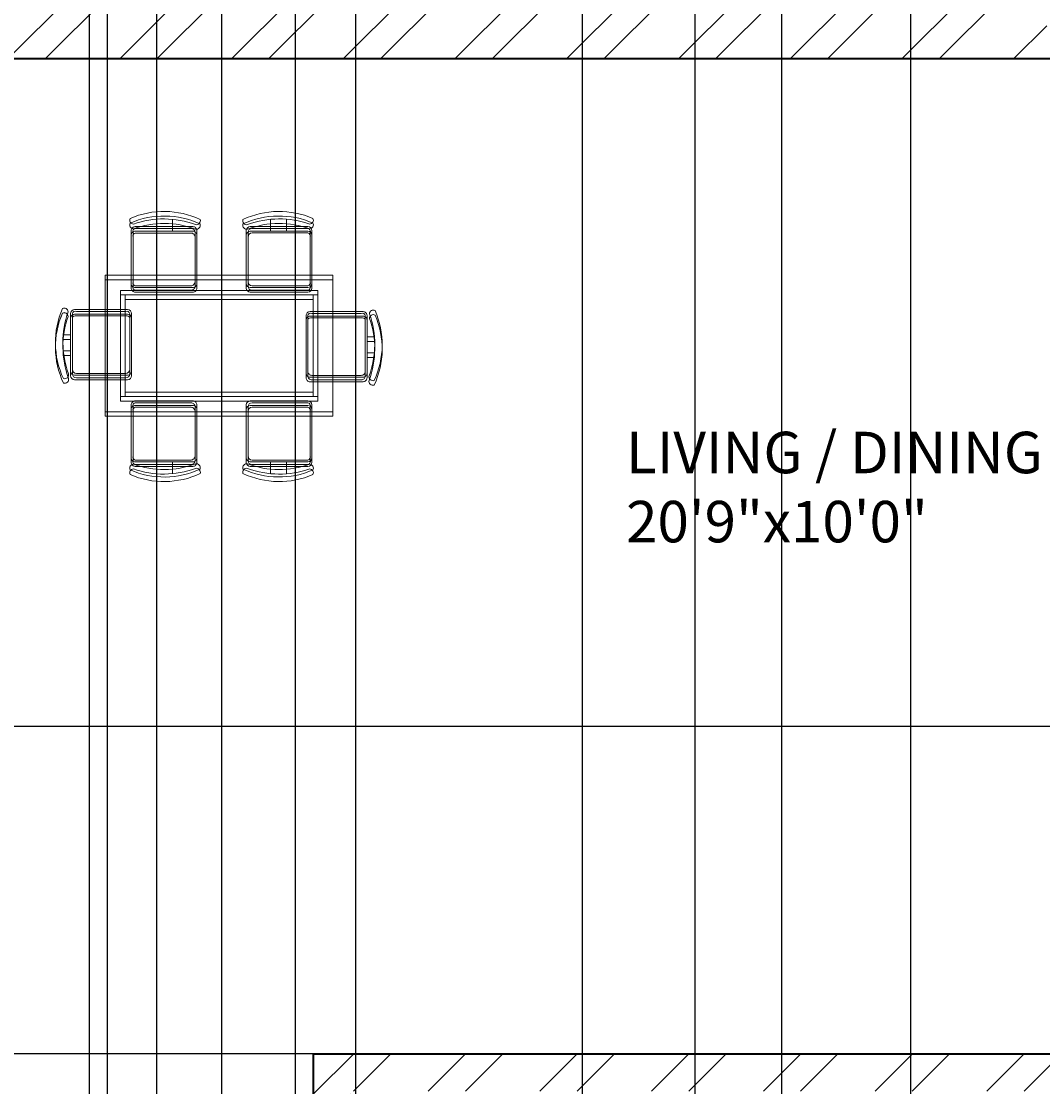
# Model space of a CAD drawing. Units: inches. Extents: x 1748 to 2382, y 1346 to 2284.
# Tile 6 of 26: x 2024 to 2147, y 1602 to 1730. Entities that reach past the tile are written whole.
import ezdxf

# ---------------------------------------------------------------- set-up
doc = ezdxf.new("R2010")
doc.units = ezdxf.units.IN
for name, color, linetype, lineweight in [('A-ANNO-DIMS', 2, 'Continuous', 18), ('A-AREA-IDEN', 7, 'Continuous', 18), ('A-FURN', 8, 'Continuous', 13), ('A-WALL', 7, 'Continuous', 35), ('A-WALL-PATT', 9, 'Continuous', 13)]:
    doc.layers.add(name, color=color, linetype=linetype, lineweight=lineweight)
doc.styles.get("Standard").update_dxf_attribs({"font": 'arial.ttf'})
doc.dimstyles.get("Standard").update_dxf_attribs({"dimtxt": 0.18, "dimasz": 0.18, "dimexe": 0.18, "dimexo": 0.0625, "dimgap": 0.09, "dimtad": 0, "dimtih": 1, "dimtoh": 1, "dimdec": 4, "dimzin": 0, "dimdsep": 46, "dimtxsty": 'Standard', "dimcen": 0.09, "dimadec": 0, "dimazin": 0, "dimtfac": 1, "dimtdec": 4, "dimtofl": 0, "dimtmove": 0, "dimatfit": 3, "dimfxl": 1, "dimtolj": 1, "dimtzin": 0, "dimarcsym": 0})

# ---------------------------------------------------------------- blocks, each defined once
blk = doc.blocks.new('TABLE-DINING')
for points in [[(0, 17.02), (27.45, 17.02), (27.45, 0.55), (0, 0.55)], [(0, 17.02), (27.45, 17.02), (27.45, 0.55), (0, 0.55)], [(0, 16.47), (27.45, 16.47), (27.45, 0), (0, 0)], [(0, 16.47), (27.45, 16.47), (27.45, 0), (0, 0)], [(1.83, 15.19), (25.62, 15.19), (25.62, 2.38), (1.83, 2.38)], [(1.83, 15.19), (25.62, 15.19), (25.62, 2.38), (1.83, 2.38)], [(1.83, 14.64), (25.62, 14.64), (25.62, 1.83), (1.83, 1.83)], [(1.83, 14.64), (25.62, 14.64), (25.62, 1.83), (1.83, 1.83)], [(2.38, 14.64), (25.07, 14.64), (25.07, 2.93), (2.38, 2.93)], [(2.38, 14.64), (25.07, 14.64), (25.07, 2.93), (2.38, 2.93)], [(2.38, 14.09), (25.07, 14.09), (25.07, 2.38), (2.38, 2.38)], [(2.38, 14.09), (25.07, 14.09), (25.07, 2.38), (2.38, 2.38)]]:
    blk.add_lwpolyline(points, close=True)
blk = doc.blocks.new('CHAIR-DINING-SIDE')
for points in [[(0.45, 8.2, -0.175809), (7.92, 8.14, 0.578392), (8.49, 8.77, 0.214524), (0.05, 8.88, 0.552014), (0.45, 8.2, -0.065079)], [(0.45, 8.2, -0.175809), (7.92, 8.14, 0.578392), (8.49, 8.77, 0.214524), (0.05, 8.88, 0.552014), (0.45, 8.2, -0.065079)], [(0.45, 7.65, -0.175809), (7.92, 7.6, 0.578392), (8.49, 8.22, 0.214524), (0.05, 8.33, 0.552014), (0.45, 7.65, -0.065079)], [(0.45, 7.65, -0.175809), (7.92, 7.6, 0.578392), (8.49, 8.22, 0.214524), (0.05, 8.33, 0.552014), (0.45, 7.65, -0.065079)], [(7.61, 7.9), (0.67, 7.9, 0.414214), (0.18, 7.42), (0.18, 1.03, 0.414214), (0.67, 0.55), (7.61, 0.55, 0.414214), (8.09, 1.03), (8.09, 7.42, 0.414214), (7.61, 7.9)], [(7.61, 7.9), (0.67, 7.9, 0.414214), (0.18, 7.42), (0.18, 1.03, 0.414214), (0.67, 0.55), (7.61, 0.55, 0.414214), (8.09, 1.03), (8.09, 7.42, 0.414214), (7.61, 7.9)], [(5.17, 7.9), (5.17, 8.78, -0.064759)], [(5.17, 7.9), (5.17, 8.78, -0.064759)], [(5.17, 7.35), (5.17, 8.23, -0.064759)], [(5.17, 7.35), (5.17, 8.23, -0.064759)], [(7.61, 7.35), (0.67, 7.35, 0.414214), (0.18, 6.87), (0.18, 0.49, 0.414214), (0.67, 0), (7.61, 0, 0.414214), (8.09, 0.49), (8.09, 6.87, 0.414214), (7.61, 7.35)], [(7.61, 7.35), (0.67, 7.35, 0.414214), (0.18, 6.87), (0.18, 0.49, 0.414214), (0.67, 0), (7.61, 0, 0.414214), (8.09, 0.49), (8.09, 6.87, 0.414214), (7.61, 7.35)]]:
    blk.add_lwpolyline(points, format="xyb")
for points in [[(3.23, 8.79), (3.23, 7.9)], [(3.23, 8.79), (3.23, 7.9)], [(3.23, 8.25), (3.23, 7.35)], [(3.23, 8.25), (3.23, 7.35)]]:
    blk.add_lwpolyline(points)
for points in [[(0.67, 7.68), (7.39, 7.68, -0.414214), (7.87, 7.2), (7.87, 1.25, -0.414214), (7.39, 0.77), (0.67, 0.77, -0.512069), (0.4, 1.25), (0.4, 7.2, -0.512069)], [(0.67, 7.68), (7.39, 7.68, -0.414214), (7.87, 7.2), (7.87, 1.25, -0.414214), (7.39, 0.77), (0.67, 0.77, -0.512069), (0.4, 1.25), (0.4, 7.2, -0.512069)], [(0.67, 7.13), (7.39, 7.13, -0.414214), (7.87, 6.65), (7.87, 0.7, -0.414214), (7.39, 0.22), (0.67, 0.22, -0.512069), (0.4, 0.7), (0.4, 6.65, -0.512069)], [(0.67, 7.13), (7.39, 7.13, -0.414214), (7.87, 6.65), (7.87, 0.7, -0.414214), (7.39, 0.22), (0.67, 0.22, -0.512069), (0.4, 0.7), (0.4, 6.65, -0.512069)]]:
    blk.add_lwpolyline(points, format="xyb", close=True)
blk = doc.blocks.new('CHAIR-DINING-END')
for points in [[(7.65, 8.61, -0.175809), (7.6, 1.14, 0.578392), (8.22, 0.57, 0.214524), (8.33, 9.01, 0.552014), (7.65, 8.61, -0.065079)], [(7.65, 8.61, -0.175809), (7.6, 1.14, 0.578392), (8.22, 0.57, 0.214524), (8.33, 9.01, 0.552014), (7.65, 8.61, -0.065079)], [(7.35, 8.4, 0.414214), (6.87, 8.88), (0.49, 8.88, 0.414214), (0, 8.4), (0, 1.46, 0.414214), (0.49, 0.97), (6.87, 0.97, 0.414214), (7.35, 1.46), (7.35, 8.4)], [(7.35, 8.4, 0.414214), (6.87, 8.88), (0.49, 8.88, 0.414214), (0, 8.4), (0, 1.46, 0.414214), (0.49, 0.97), (6.87, 0.97, 0.414214), (7.35, 1.46), (7.35, 8.4)], [(7.35, 7.85, 0.414214), (6.87, 8.33), (0.49, 8.33, 0.414214), (0, 7.85), (0, 0.91, 0.414214), (0.49, 0.42), (6.87, 0.42, 0.414214), (7.35, 0.91), (7.35, 7.85)], [(7.35, 7.85, 0.414214), (6.87, 8.33), (0.49, 8.33, 0.414214), (0, 7.85), (0, 0.91, 0.414214), (0.49, 0.42), (6.87, 0.42, 0.414214), (7.35, 0.91), (7.35, 7.85)], [(7.65, 8.06, -0.175809), (7.6, 0.59, 0.578392), (8.22, 0.02, 0.214524), (8.33, 8.46, 0.552014), (7.65, 8.06, -0.065079)], [(7.65, 8.06, -0.175809), (7.6, 0.59, 0.578392), (8.22, 0.02, 0.214524), (8.33, 8.46, 0.552014), (7.65, 8.06, -0.065079)], [(7.35, 3.89), (8.23, 3.89, -0.064759)], [(7.35, 3.89), (8.23, 3.89, -0.064759)], [(7.35, 3.34), (8.23, 3.34, -0.064759)], [(7.35, 3.34), (8.23, 3.34, -0.064759)]]:
    blk.add_lwpolyline(points, format="xyb")
for points in [[(7.13, 8.39), (7.13, 1.67, -0.414214), (6.65, 1.19), (0.7, 1.19, -0.414214), (0.22, 1.67), (0.22, 8.39, -0.512069), (0.7, 8.66), (6.65, 8.66, -0.512069)], [(7.13, 8.39), (7.13, 1.67, -0.414214), (6.65, 1.19), (0.7, 1.19, -0.414214), (0.22, 1.67), (0.22, 8.39, -0.512069), (0.7, 8.66), (6.65, 8.66, -0.512069)], [(7.13, 7.84), (7.13, 1.13, -0.414214), (6.65, 0.64), (0.7, 0.64, -0.414214), (0.22, 1.13), (0.22, 7.84, -0.512069), (0.7, 8.11), (6.65, 8.11, -0.512069)], [(7.13, 7.84), (7.13, 1.12, -0.414214), (6.65, 0.64), (0.7, 0.64, -0.414214), (0.22, 1.12), (0.22, 7.84, -0.512069), (0.7, 8.11), (6.65, 8.11, -0.512069)]]:
    blk.add_lwpolyline(points, format="xyb", close=True)
for points in [[(8.25, 5.84), (7.35, 5.84)], [(8.25, 5.84), (7.35, 5.84)], [(8.25, 5.29), (7.35, 5.29)], [(8.25, 5.29), (7.35, 5.29)]]:
    blk.add_lwpolyline(points)
blk = doc.blocks.new('*D36')
at = {"layer": 'A-ANNO-DIMS', "color": 0, "lineweight": -2, "transparency": 16777216}
for p, q in [((2031.96, 1970.29), (2031.96, 1360.47)), ((2130.96, 1970.29), (2130.96, 1360.47)), ((2032.14, 1360.65), (2081.24, 1360.65)), ((2130.78, 1360.65), (2081.68, 1360.65))]:
    blk.add_line(p, q, dxfattribs=at)
at = {"layer": 'A-ANNO-DIMS', "color": 0, "transparency": 16777216}
for points in [[(2032.14, 1360.68), (2032.14, 1360.62), (2031.96, 1360.65)], [(2130.78, 1360.68), (2130.78, 1360.62), (2130.96, 1360.65)]]:
    blk.add_solid(points, dxfattribs=at)
at = {"layer": 'Defpoints', "color": 0, "transparency": 16777216}
for p in [(2031.96, 1970.35), (2130.96, 1970.35), (2130.96, 1360.65)]:
    blk.add_point(p, dxfattribs=at)
at = {"layer": 'A-ANNO-DIMS', "color": 0, "transparency": 16777216, "insert": (2081.46, 1360.65), "char_height": 0.18, "attachment_point": 5}
blk.add_mtext('\\A1;99', dxfattribs=at)
blk = doc.blocks.new('*D51')
at = {"layer": 'A-ANNO-DIMS', "color": 0, "lineweight": -2, "transparency": 16777216}
for p, q in [((1968.44, 2223.79), (1968.44, 1360.47)), ((2040.07, 2223.79), (2040.07, 1360.47)), ((1968.62, 1360.65), (2003.86, 1360.65)), ((2039.89, 1360.65), (2004.65, 1360.65))]:
    blk.add_line(p, q, dxfattribs=at)
at = {"layer": 'A-ANNO-DIMS', "color": 0, "transparency": 16777216}
for points in [[(1968.62, 1360.68), (1968.62, 1360.62), (1968.44, 1360.65)], [(2039.89, 1360.68), (2039.89, 1360.62), (2040.07, 1360.65)]]:
    blk.add_solid(points, dxfattribs=at)
at = {"layer": 'Defpoints', "color": 0, "transparency": 16777216}
for p in [(1968.44, 2223.85), (2040.07, 2223.85), (2040.07, 1360.65)]:
    blk.add_point(p, dxfattribs=at)
at = {"layer": 'A-ANNO-DIMS', "color": 0, "transparency": 16777216, "insert": (2004.26, 1360.65), "char_height": 0.18, "attachment_point": 5}
blk.add_mtext('\\A1;71.62', dxfattribs=at)
blk = doc.blocks.new('*D52')
at = {"layer": 'A-ANNO-DIMS', "color": 0, "lineweight": -2, "transparency": 16777216}
for p, q in [((2064.07, 2223.79), (2064.07, 1360.47)), ((2091.4, 2223.79), (2091.4, 1360.47)), ((2064.25, 1360.65), (2077.34, 1360.65)), ((2091.22, 1360.65), (2078.13, 1360.65))]:
    blk.add_line(p, q, dxfattribs=at)
at = {"layer": 'A-ANNO-DIMS', "color": 0, "transparency": 16777216}
for points in [[(2064.25, 1360.68), (2064.25, 1360.62), (2064.07, 1360.65)], [(2091.22, 1360.68), (2091.22, 1360.62), (2091.4, 1360.65)]]:
    blk.add_solid(points, dxfattribs=at)
at = {"layer": 'Defpoints', "color": 0, "transparency": 16777216}
for p in [(2064.07, 2223.85), (2091.4, 2223.85), (2091.4, 1360.65)]:
    blk.add_point(p, dxfattribs=at)
at = {"layer": 'A-ANNO-DIMS', "color": 0, "transparency": 16777216, "insert": (2077.73, 1360.65), "char_height": 0.18, "attachment_point": 5}
blk.add_mtext('\\A1;27.33', dxfattribs=at)
blk = doc.blocks.new('*D53')
at = {"layer": 'A-ANNO-DIMS', "color": 0, "lineweight": -2, "transparency": 16777216}
for p, q in [((2115.4, 2223.79), (2115.4, 1360.47)), ((2167.02, 2223.79), (2167.02, 1360.47)), ((2115.58, 1360.65), (2140.81, 1360.65)), ((2166.84, 1360.65), (2141.6, 1360.65))]:
    blk.add_line(p, q, dxfattribs=at)
at = {"layer": 'A-ANNO-DIMS', "color": 0, "transparency": 16777216}
for points in [[(2115.58, 1360.68), (2115.58, 1360.62), (2115.4, 1360.65)], [(2166.84, 1360.68), (2166.84, 1360.62), (2167.02, 1360.65)]]:
    blk.add_solid(points, dxfattribs=at)
at = {"layer": 'Defpoints', "color": 0, "transparency": 16777216}
for p in [(2115.4, 2223.85), (2167.02, 2223.85), (2167.02, 1360.65)]:
    blk.add_point(p, dxfattribs=at)
at = {"layer": 'A-ANNO-DIMS', "color": 0, "transparency": 16777216, "insert": (2141.21, 1360.65), "char_height": 0.18, "attachment_point": 5}
blk.add_mtext('\\A1;51.62', dxfattribs=at)
blk = doc.blocks.new('*D55')
at = {"layer": 'A-ANNO-DIMS', "color": 0, "lineweight": -2, "transparency": 16777216}
for p, q in [((2288.4, 1645.3), (1779.88, 1645.3)), ((1780.06, 1645.12), (1780.06, 1625.76)), ((1780.06, 1606.03), (1780.06, 1625.39)), ((2288.4, 1605.85), (1779.88, 1605.85))]:
    blk.add_line(p, q, dxfattribs=at)
at = {"layer": 'A-ANNO-DIMS', "color": 0, "transparency": 16777216}
for points in [[(1780.03, 1645.12), (1780.09, 1645.12), (1780.06, 1645.3)], [(1780.03, 1606.03), (1780.09, 1606.03), (1780.06, 1605.85)]]:
    blk.add_solid(points, dxfattribs=at)
at = {"layer": 'Defpoints', "color": 0, "transparency": 16777216}
for p in [(1780.06, 1645.3), (2288.46, 1645.3), (2288.46, 1605.85)]:
    blk.add_point(p, dxfattribs=at)
at = {"layer": 'A-ANNO-DIMS', "color": 0, "transparency": 16777216, "insert": (1780.06, 1625.58), "char_height": 0.18, "attachment_point": 5}
blk.add_mtext('\\A1;39.454', dxfattribs=at)
blk = doc.blocks.new('*D61')
at = {"layer": 'A-ANNO-DIMS', "color": 0, "lineweight": -2, "transparency": 16777216}
for p, q in [((2047.92, 1854.79), (2047.92, 1360.47)), ((2104.96, 1854.79), (2104.96, 1360.47)), ((2048.1, 1360.65), (2076.04, 1360.65)), ((2104.78, 1360.65), (2076.83, 1360.65))]:
    blk.add_line(p, q, dxfattribs=at)
at = {"layer": 'A-ANNO-DIMS', "color": 0, "transparency": 16777216}
for points in [[(2048.1, 1360.68), (2048.1, 1360.62), (2047.92, 1360.65)], [(2104.78, 1360.68), (2104.78, 1360.62), (2104.96, 1360.65)]]:
    blk.add_solid(points, dxfattribs=at)
at = {"layer": 'Defpoints', "color": 0, "transparency": 16777216}
for p in [(2047.92, 1854.85), (2104.96, 1854.85), (2104.96, 1360.65)]:
    blk.add_point(p, dxfattribs=at)
at = {"layer": 'A-ANNO-DIMS', "color": 0, "transparency": 16777216, "insert": (2076.44, 1360.65), "char_height": 0.18, "attachment_point": 5}
blk.add_mtext('\\A1;57.04', dxfattribs=at)
blk = doc.blocks.new('*D78')
at = {"layer": 'A-ANNO-DIMS', "color": 0, "lineweight": -2, "transparency": 16777216}
for p, q in [((2034.13, 2132.54), (2034.13, 1360.47)), ((2056.8, 2127.06), (2056.8, 1360.47)), ((2034.31, 1360.65), (2045, 1360.65)), ((2056.62, 1360.65), (2045.93, 1360.65))]:
    blk.add_line(p, q, dxfattribs=at)
at = {"layer": 'A-ANNO-DIMS', "color": 0, "transparency": 16777216}
for points in [[(2034.31, 1360.68), (2034.31, 1360.62), (2034.13, 1360.65)], [(2056.62, 1360.68), (2056.62, 1360.62), (2056.8, 1360.65)]]:
    blk.add_solid(points, dxfattribs=at)
at = {"layer": 'Defpoints', "color": 0, "transparency": 16777216}
for p in [(2034.13, 2132.6), (2056.8, 2127.13), (2056.8, 1360.65)]:
    blk.add_point(p, dxfattribs=at)
at = {"layer": 'A-ANNO-DIMS', "color": 0, "transparency": 16777216, "insert": (2045.47, 1360.65), "char_height": 0.18, "attachment_point": 5}
blk.add_mtext('\\A1;22.663', dxfattribs=at)

msp = doc.modelspace()

# ---------------------------------------------------------------- hatches: boundary and pattern name
at = {"layer": 'A-WALL-PATT'}
h = msp.add_hatch(dxfattribs=at)
h.set_pattern_fill('ANSI32', color=256)
h.paths.add_polyline_path([(1908.4445, 2232.8497), (1821.9607, 2232.8497), (1821.9607, 2223.8497), (1865.4607, 2223.8497), (1865.4607, 2209.9185), (1869.9607, 2209.9185), (1869.9607, 2223.8497), (1908.4445, 2223.8497), (1908.4445, 2228.3497)])
h.paths.add_polyline_path([(2040.0683, 2232.8497), (1968.4445, 2232.8497), (1968.4445, 2223.8497), (2025.9607, 2223.8497), (2025.9607, 2130.3497), (2032.1341, 2130.3497), (2032.1341, 2132.5997), (2032.1341, 2134.8497), (2030.4607, 2134.8497), (2030.4607, 2223.8497), (2040.0683, 2223.8497)])
h.paths.add_polyline_path([(2091.3969, 2232.8497), (2064.0683, 2232.8497), (2064.0683, 2223.8497), (2078.4607, 2223.8497), (2078.4607, 2134.8497), (2051.1563, 2134.8497), (2051.1563, 2130.3497), (2078.4607, 2130.3497), (2078.4607, 2128.6813), (2082.9607, 2128.6813), (2082.9607, 2130.3497), (2086.1879, 2130.3497), (2086.1879, 2132.5997), (2086.1879, 2134.8497), (2082.9607, 2134.8497), (2082.9607, 2223.8497), (2091.3969, 2223.8497), (2091.3969, 2228.3497)])
h.paths.add_polyline_path([(2167.0164, 2232.8497), (2115.3969, 2232.8497), (2115.3969, 2223.8497), (2130.9607, 2223.8497), (2130.9607, 2134.8497), (2106.9607, 2134.8497), (2106.9607, 2130.3497), (2135.4607, 2130.3497), (2135.4607, 2223.8497), (2167.0164, 2223.8497), (2167.0164, 2228.3497)])
h.paths.add_polyline_path([(1869.9607, 2149.9185), (1865.4607, 2149.9185), (1865.4607, 2127.8942), (1869.9607, 2127.8942)])
h.paths.add_polyline_path([(2082.9607, 2104.4871), (2080.7107, 2104.4871), (2078.4607, 2104.4871), (2078.4607, 2103.8497), (1869.9607, 2103.8497), (1869.9607, 2108.6062), (1867.7107, 2108.6062), (1865.4607, 2108.6062), (1865.4607, 2103.8497), (1821.9607, 2103.8497), (1821.9607, 2099.3497), (1865.4607, 2099.3497), (1865.4607, 2094.7509), (1869.9607, 2094.7509), (1869.9607, 2099.3497), (2025.9607, 2099.3497), (2025.9607, 2096.4326), (2030.4607, 2096.4326), (2030.4607, 2099.3497), (2082.9607, 2099.3497)])
h.paths.add_polyline_path([(1928.9457, 1401.1212), (2176.8693, 1401.1212), (2176.8693, 1438.214), (1928.9457, 1438.214)], flags=9)
h.paths.add_polyline_path([(2122.2668, 2048.1927), (2177.9387, 2048.1927), (2177.9387, 2066.85), (2122.2668, 2066.85)], flags=9)
h.paths.add_polyline_path([(2272.688, 2153.8197), (2272.688, 2216.746), (2262.3845, 2216.746), (2262.3845, 2153.8197)], flags=9)
h.paths.add_polyline_path([(2157.2928, 2166.5593), (2196.3822, 2166.5593), (2196.3822, 2185.2167), (2157.2928, 2185.2167)], flags=9)
h.paths.add_polyline_path([(2089.3407, 2162.0698), (2124.3987, 2162.0698), (2124.3987, 2180.7272), (2089.3407, 2180.7272)], flags=9)
h.paths.add_polyline_path([(2037.4521, 2160.0913), (2072.5101, 2160.0913), (2072.5101, 2178.7486), (2037.4521, 2178.7486)], flags=9)
h.paths.add_polyline_path([(1884.7894, 2104.1554), (1923.6297, 2104.1554), (1923.6297, 2122.8127), (1884.7894, 2122.8127)], flags=9)
h.paths.add_polyline_path([(1851.2832, 2142.9749), (1851.2832, 2199.3051), (1840.9796, 2199.3051), (1840.9796, 2142.9749)], flags=9)
h.paths.add_polyline_path([(1844.8763, 2017.2834), (1844.8763, 2073.6136), (1834.5728, 2073.6136), (1834.5728, 2017.2834)], flags=9)
h.paths.add_polyline_path([(1897.1577, 2073.1279), (1935.9981, 2073.1279), (1935.9981, 2091.7853), (1897.1577, 2091.7853)], flags=9)
h.paths.add_polyline_path([(1952.3395, 1802.4231), (2008.0114, 1802.4231), (2008.0114, 1821.0805), (1952.3395, 1821.0805)], flags=9)
h.paths.add_polyline_path([(1978.8184, 1857.6841), (2017.7338, 1857.6841), (2017.7338, 1876.3415), (1978.8184, 1876.3415)], flags=9)
h.paths.add_polyline_path([(1979.6513, 1925.9516), (2008.8089, 1925.9516), (2008.8089, 1944.6089), (1979.6513, 1944.6089)], flags=9)
h.paths.add_polyline_path([(1838.5553, 1860.3527), (1877.3957, 1860.3527), (1877.3957, 1879.01), (1838.5553, 1879.01)], flags=9)
h.paths.add_polyline_path([(1883.9018, 1787.3013), (1883.9018, 1843.6315), (1873.5983, 1843.6315), (1873.5983, 1787.3013)], flags=9)
h.paths.add_polyline_path([(1873.7079, 1509.1938), (1873.7079, 1583.7709), (1863.4044, 1583.7709), (1863.4044, 1509.1938)], flags=9)
h.paths.add_polyline_path([(1916.2259, 1603.3681), (1955.0663, 1603.3681), (1955.0663, 1622.0254), (1916.2259, 1622.0254)], flags=9)
h.paths.add_polyline_path([(1876.3013, 1636.757), (1876.3013, 1693.0871), (1865.9978, 1693.0871), (1865.9978, 1636.757)], flags=9)
h.paths.add_polyline_path([(1921.3138, 1521.8316), (1964.0662, 1521.8316), (1964.0662, 1540.489), (1921.3138, 1540.489)], flags=9)
h.paths.add_polyline_path([(2017.5657, 1497.5078), (2046.7983, 1497.5078), (2046.7983, 1516.1651), (2017.5657, 1516.1651)], flags=9)
h.paths.add_polyline_path([(2066.8661, 1499.3902), (2096.0988, 1499.3902), (2096.0988, 1518.0475), (2066.8661, 1518.0475)], flags=9)
h.paths.add_polyline_path([(2155.4835, 1571.6596), (2198.2358, 1571.6596), (2198.2358, 1590.3169), (2155.4835, 1590.3169)], flags=9)
h.paths.add_polyline_path([(2094.9136, 1664.6812), (2150.5855, 1664.6812), (2150.5855, 1683.3386), (2094.9136, 1683.3386)], flags=9)
h.paths.add_polyline_path([(2257.6902, 1863.1628), (2269.8935, 1863.1628), (2269.8935, 1873.4664), (2257.6902, 1873.4664)], flags=9)
h.paths.add_polyline_path([(2164.0748, 1880.3089), (2189.8694, 1880.3089), (2189.8694, 1890.6124), (2164.0748, 1890.6124)], flags=9)
h.paths.add_polyline_path([(2239.4394, 1931.0585), (2268.8187, 1931.0585), (2268.8187, 1949.7159), (2239.4394, 1949.7159)], flags=9)
h = msp.add_hatch(dxfattribs=at)
h.set_pattern_fill('ANSI32', color=256)
h.paths.add_polyline_path([(2297.4607, 2232.8497), (2203.0164, 2232.8497), (2203.0164, 2223.8497), (2244.9607, 2223.8497), (2244.9607, 2127.8554), (2249.4607, 2127.8554), (2249.4607, 2223.8497), (2297.4607, 2223.8497)])
h.paths.add_polyline_path([(2297.4607, 2103.8497), (2249.4607, 2103.8497), (2249.4607, 2106.7497), (2247.2107, 2106.7497), (2244.9607, 2106.7497), (2244.9607, 2103.8497), (2130.9607, 2103.8497), (2130.9607, 2099.3497), (2288.4607, 2099.3497), (2288.4607, 2077.2008), (2297.4607, 2077.2008)])
h.paths.add_polyline_path([(1928.9457, 1401.1212), (2176.8693, 1401.1212), (2176.8693, 1438.214), (1928.9457, 1438.214)], flags=9)
h.paths.add_polyline_path([(2122.2668, 2048.1927), (2177.9387, 2048.1927), (2177.9387, 2066.85), (2122.2668, 2066.85)], flags=9)
h.paths.add_polyline_path([(2272.688, 2153.8197), (2272.688, 2216.746), (2262.3845, 2216.746), (2262.3845, 2153.8197)], flags=25)
h.paths.add_polyline_path([(2157.2928, 2166.5593), (2196.3822, 2166.5593), (2196.3822, 2185.2167), (2157.2928, 2185.2167)], flags=9)
h.paths.add_polyline_path([(2089.3407, 2162.0698), (2124.3987, 2162.0698), (2124.3987, 2180.7272), (2089.3407, 2180.7272)], flags=9)
h.paths.add_polyline_path([(2037.4521, 2160.0913), (2072.5101, 2160.0913), (2072.5101, 2178.7486), (2037.4521, 2178.7486)], flags=9)
h.paths.add_polyline_path([(1884.7894, 2104.1554), (1923.6297, 2104.1554), (1923.6297, 2122.8127), (1884.7894, 2122.8127)], flags=9)
h.paths.add_polyline_path([(1851.2832, 2142.9749), (1851.2832, 2199.3051), (1840.9796, 2199.3051), (1840.9796, 2142.9749)], flags=9)
h.paths.add_polyline_path([(1844.8763, 2017.2834), (1844.8763, 2073.6136), (1834.5728, 2073.6136), (1834.5728, 2017.2834)], flags=9)
h.paths.add_polyline_path([(1897.1577, 2073.1279), (1935.9981, 2073.1279), (1935.9981, 2091.7853), (1897.1577, 2091.7853)], flags=9)
h.paths.add_polyline_path([(1952.3395, 1802.4231), (2008.0114, 1802.4231), (2008.0114, 1821.0805), (1952.3395, 1821.0805)], flags=9)
h.paths.add_polyline_path([(1978.8184, 1857.6841), (2017.7338, 1857.6841), (2017.7338, 1876.3415), (1978.8184, 1876.3415)], flags=9)
h.paths.add_polyline_path([(1979.6513, 1925.9516), (2008.8089, 1925.9516), (2008.8089, 1944.6089), (1979.6513, 1944.6089)], flags=9)
h.paths.add_polyline_path([(1838.5553, 1860.3527), (1877.3957, 1860.3527), (1877.3957, 1879.01), (1838.5553, 1879.01)], flags=9)
h.paths.add_polyline_path([(1883.9018, 1787.3013), (1883.9018, 1843.6315), (1873.5983, 1843.6315), (1873.5983, 1787.3013)], flags=9)
h.paths.add_polyline_path([(1873.7079, 1509.1938), (1873.7079, 1583.7709), (1863.4044, 1583.7709), (1863.4044, 1509.1938)], flags=9)
h.paths.add_polyline_path([(1916.2259, 1603.3681), (1955.0663, 1603.3681), (1955.0663, 1622.0254), (1916.2259, 1622.0254)], flags=9)
h.paths.add_polyline_path([(1876.3013, 1636.757), (1876.3013, 1693.0871), (1865.9978, 1693.0871), (1865.9978, 1636.757)], flags=9)
h.paths.add_polyline_path([(1921.3138, 1521.8316), (1964.0662, 1521.8316), (1964.0662, 1540.489), (1921.3138, 1540.489)], flags=9)
h.paths.add_polyline_path([(2017.5657, 1497.5078), (2046.7983, 1497.5078), (2046.7983, 1516.1651), (2017.5657, 1516.1651)], flags=9)
h.paths.add_polyline_path([(2066.8661, 1499.3902), (2096.0988, 1499.3902), (2096.0988, 1518.0475), (2066.8661, 1518.0475)], flags=9)
h.paths.add_polyline_path([(2155.4835, 1571.6596), (2198.2358, 1571.6596), (2198.2358, 1590.3169), (2155.4835, 1590.3169)], flags=9)
h.paths.add_polyline_path([(2094.9136, 1664.6812), (2150.5855, 1664.6812), (2150.5855, 1683.3386), (2094.9136, 1683.3386)], flags=9)
h.paths.add_polyline_path([(2257.6902, 1863.1628), (2269.8935, 1863.1628), (2269.8935, 1873.4664), (2257.6902, 1873.4664)], flags=9)
h.paths.add_polyline_path([(2164.0748, 1880.3089), (2189.8694, 1880.3089), (2189.8694, 1890.6124), (2164.0748, 1890.6124)], flags=9)
h.paths.add_polyline_path([(2239.4394, 1931.0585), (2268.8187, 1931.0585), (2268.8187, 1949.7159), (2239.4394, 1949.7159)], flags=9)
h = msp.add_hatch(dxfattribs=at)
h.set_pattern_fill('ANSI32', color=256)
h.paths.add_polyline_path([(1919.6777, 1476.8497), (1900.6426, 1476.8497), (1900.6426, 1522.0826), (1898.3926, 1522.0826), (1896.1426, 1522.0826), (1896.1426, 1476.8497), (1857.1426, 1476.8497), (1857.1426, 1467.8497), (1896.1426, 1467.8497), (1919.6777, 1467.8497), (1919.6777, 1472.3497)])
h.paths.add_polyline_path([(2018.7873, 1472.3497), (2018.7873, 1476.8497), (2010.9607, 1476.8497), (2010.9607, 1560.8497), (2034.9607, 1560.8497), (2034.9607, 1565.3497), (2006.4607, 1565.3497), (2006.4607, 1476.8497), (1955.6777, 1476.8497), (1955.6777, 1467.8497), (2018.7873, 1467.8497)])
h.paths.add_polyline_path([(2152.3354, 1472.3497), (2152.3354, 1476.8497), (2115.9607, 1476.8497), (2115.9607, 1565.3497), (2109.2204, 1565.3497), (2109.2204, 1563.0997), (2109.2204, 1560.8497), (2111.4607, 1560.8497), (2111.4607, 1476.8497), (2095.3617, 1476.8497), (2095.3617, 1467.8497), (2152.3354, 1467.8497)])
h.paths.add_polyline_path([(2071.3617, 1476.8497), (2063.4607, 1476.8497), (2063.4607, 1560.8497), (2090.1865, 1560.8497), (2090.1865, 1565.3497), (2063.4607, 1565.3497), (2063.4607, 1572.5485), (2061.2107, 1572.5485), (2058.9607, 1572.5485), (2058.9607, 1565.3497), (2055.6281, 1565.3497), (2055.6281, 1560.8497), (2058.9607, 1560.8497), (2058.9607, 1476.8497), (2042.7873, 1476.8497), (2042.7873, 1467.8497), (2071.3617, 1467.8497), (2071.3617, 1472.3497)])
h.paths.add_polyline_path([(2297.4607, 1506.5652), (2288.4607, 1506.5652), (2288.4607, 1476.8497), (2212.3354, 1476.8497), (2212.3354, 1467.8497), (2297.4607, 1467.8497)])
h.paths.add_polyline_path([(2297.4607, 1645.3038), (2288.4607, 1645.3038), (2288.4607, 1605.8497), (2058.9607, 1605.8497), (2058.9607, 1600.1857), (2061.2107, 1600.1857), (2063.4607, 1600.1857), (2063.4607, 1601.3497), (2288.4607, 1601.3497), (2288.4607, 1566.5652), (2297.4607, 1566.5652)])
h.paths.add_polyline_path([(2010.9607, 1609.0561), (2008.7107, 1609.0561), (2006.4607, 1609.0561), (2006.4607, 1605.8497), (1900.6426, 1605.8497), (1900.6426, 1609.7171), (1898.3926, 1609.7171), (1896.1426, 1609.7171), (1896.1426, 1605.8497), (1857.1426, 1605.8497), (1857.1426, 1601.3497), (1896.1426, 1601.3497), (1896.1426, 1542.5447), (1900.6426, 1542.5447), (1900.6426, 1601.3497), (2010.9607, 1601.3497)])
h.paths.add_polyline_path([(1928.9457, 1401.1212), (2176.8693, 1401.1212), (2176.8693, 1438.214), (1928.9457, 1438.214)], flags=9)
h.paths.add_polyline_path([(2122.2668, 2048.1927), (2177.9387, 2048.1927), (2177.9387, 2066.85), (2122.2668, 2066.85)], flags=9)
h.paths.add_polyline_path([(2272.688, 2153.8197), (2272.688, 2216.746), (2262.3845, 2216.746), (2262.3845, 2153.8197)], flags=9)
h.paths.add_polyline_path([(2157.2928, 2166.5593), (2196.3822, 2166.5593), (2196.3822, 2185.2167), (2157.2928, 2185.2167)], flags=9)
h.paths.add_polyline_path([(2089.3407, 2162.0698), (2124.3987, 2162.0698), (2124.3987, 2180.7272), (2089.3407, 2180.7272)], flags=9)
h.paths.add_polyline_path([(2037.4521, 2160.0913), (2072.5101, 2160.0913), (2072.5101, 2178.7486), (2037.4521, 2178.7486)], flags=9)
h.paths.add_polyline_path([(1884.7894, 2104.1554), (1923.6297, 2104.1554), (1923.6297, 2122.8127), (1884.7894, 2122.8127)], flags=9)
h.paths.add_polyline_path([(1851.2832, 2142.9749), (1851.2832, 2199.3051), (1840.9796, 2199.3051), (1840.9796, 2142.9749)], flags=9)
h.paths.add_polyline_path([(1844.8763, 2017.2834), (1844.8763, 2073.6136), (1834.5728, 2073.6136), (1834.5728, 2017.2834)], flags=9)
h.paths.add_polyline_path([(1897.1577, 2073.1279), (1935.9981, 2073.1279), (1935.9981, 2091.7853), (1897.1577, 2091.7853)], flags=9)
h.paths.add_polyline_path([(1952.3395, 1802.4231), (2008.0114, 1802.4231), (2008.0114, 1821.0805), (1952.3395, 1821.0805)], flags=9)
h.paths.add_polyline_path([(1978.8184, 1857.6841), (2017.7338, 1857.6841), (2017.7338, 1876.3415), (1978.8184, 1876.3415)], flags=9)
h.paths.add_polyline_path([(1979.6513, 1925.9516), (2008.8089, 1925.9516), (2008.8089, 1944.6089), (1979.6513, 1944.6089)], flags=9)
h.paths.add_polyline_path([(1838.5553, 1860.3527), (1877.3957, 1860.3527), (1877.3957, 1879.01), (1838.5553, 1879.01)], flags=9)
h.paths.add_polyline_path([(1883.9018, 1787.3013), (1883.9018, 1843.6315), (1873.5983, 1843.6315), (1873.5983, 1787.3013)], flags=9)
h.paths.add_polyline_path([(1873.7079, 1509.1938), (1873.7079, 1583.7709), (1863.4044, 1583.7709), (1863.4044, 1509.1938)], flags=9)
h.paths.add_polyline_path([(1916.2259, 1603.3681), (1955.0663, 1603.3681), (1955.0663, 1622.0254), (1916.2259, 1622.0254)], flags=9)
h.paths.add_polyline_path([(1876.3013, 1636.757), (1876.3013, 1693.0871), (1865.9978, 1693.0871), (1865.9978, 1636.757)], flags=9)
h.paths.add_polyline_path([(1921.3138, 1521.8316), (1964.0662, 1521.8316), (1964.0662, 1540.489), (1921.3138, 1540.489)], flags=9)
h.paths.add_polyline_path([(2017.5657, 1497.5078), (2046.7983, 1497.5078), (2046.7983, 1516.1651), (2017.5657, 1516.1651)], flags=9)
h.paths.add_polyline_path([(2066.8661, 1499.3902), (2096.0988, 1499.3902), (2096.0988, 1518.0475), (2066.8661, 1518.0475)], flags=9)
h.paths.add_polyline_path([(2155.4835, 1571.6596), (2198.2358, 1571.6596), (2198.2358, 1590.3169), (2155.4835, 1590.3169)], flags=25)
h.paths.add_polyline_path([(2094.9136, 1664.6812), (2150.5855, 1664.6812), (2150.5855, 1683.3386), (2094.9136, 1683.3386)], flags=9)
h.paths.add_polyline_path([(2257.6902, 1863.1628), (2269.8935, 1863.1628), (2269.8935, 1873.4664), (2257.6902, 1873.4664)], flags=9)
h.paths.add_polyline_path([(2164.0748, 1880.3089), (2189.8694, 1880.3089), (2189.8694, 1890.6124), (2164.0748, 1890.6124)], flags=9)
h.paths.add_polyline_path([(2239.4394, 1931.0585), (2268.8187, 1931.0585), (2268.8187, 1949.7159), (2239.4394, 1949.7159)], flags=9)
h = msp.add_hatch(dxfattribs=at)
h.set_pattern_fill('ANSI32', color=256)
h.paths.add_polyline_path([(1900.6426, 1652.723), (1896.1426, 1652.723), (1896.1426, 1629.9029), (1900.6426, 1629.9029)])
h.paths.add_polyline_path([(2206.0699, 1859.3497), (2197.0699, 1859.3497), (2197.0699, 1734.8497), (2206.0699, 1734.8497)], flags=17)
h.paths.add_polyline_path([(2297.4607, 1865.3269), (2288.4607, 1865.3269), (2288.4607, 1734.8497), (2206.0699, 1734.8497), (2180.4551, 1734.8497), (2180.4551, 1725.8497), (2197.0699, 1725.8497), (2206.0699, 1725.8497), (2288.4607, 1725.8497), (2288.4607, 1705.3038), (2297.4607, 1705.3038)])
h.paths.add_polyline_path([(2139.9607, 1815.8001), (2135.4607, 1815.8001), (2130.9607, 1815.8001), (2130.9607, 1734.8497), (1900.6426, 1734.8497), (1900.6426, 1738.9477), (1898.3926, 1738.9477), (1896.1426, 1738.9477), (1896.1426, 1734.8497), (1857.1426, 1734.8497), (1857.1426, 1725.8497), (1896.1426, 1725.8497), (1896.1426, 1712.723), (1900.6426, 1712.723), (1900.6426, 1725.8497), (2006.4607, 1725.8497), (2006.4607, 1637.448), (2010.9607, 1637.448), (2010.9607, 1725.8497), (2139.9607, 1725.8497), (2147.389, 1725.8497), (2147.389, 1730.3497), (2147.389, 1734.8497), (2139.9607, 1734.8497)])
h.paths.add_polyline_path([(2149.8497, 1917.8497), (2149.8497, 1922.3497), (2139.9607, 1922.3497), (2139.9607, 1979.3497), (2030.4607, 1979.3497), (2030.4607, 2069.8971), (2028.2107, 2069.8971), (2025.9607, 2069.8971), (2025.9607, 1979.3497), (1869.9607, 1979.3497), (1869.9607, 1998.93), (1865.4607, 1998.93), (1865.4607, 1979.3497), (1821.9607, 1979.3497), (1821.9607, 1952.7922), (1826.9306, 1952.7922), (1830.9607, 1952.7922), (1830.9607, 1970.3497), (1962.9607, 1970.3497), (1962.9607, 1926.5713), (1967.4607, 1926.5713), (1967.4607, 1970.3497), (2027.4607, 1970.3497), (2027.4607, 1898.3497), (2004.9604, 1898.3497), (2004.9604, 1893.8497), (2027.4607, 1893.8497), (2027.4607, 1859.3497), (1958.8973, 1859.3497), (1958.8973, 1854.8497), (2047.917, 1854.8497), (2047.917, 1859.3497), (2031.9607, 1859.3497), (2031.9607, 1970.3497), (2130.9607, 1970.3497), (2130.9607, 1859.3497), (2104.9565, 1859.3497), (2104.9565, 1854.8497), (2130.9607, 1854.8497), (2130.9607, 1849.0684), (2139.9607, 1849.0684), (2139.9607, 1913.3497), (2149.8497, 1913.3497)])
h.paths.add_polyline_path([(1928.9996, 1859.3497), (1830.9607, 1859.3497), (1830.9607, 1892.7922), (1821.9607, 1892.7922), (1821.9607, 1854.8497), (1896.1426, 1854.8497), (1896.1426, 1836.6443), (1898.378, 1836.6443), (1900.6426, 1836.6443), (1900.6426, 1854.8497), (1928.9996, 1854.8497), (1928.9996, 1857.0997)])
h.paths.add_polyline_path([(1980.9604, 1896.0997), (1980.9604, 1898.3497), (1967.4607, 1898.3497), (1967.4607, 1902.3846), (1962.9607, 1902.3846), (1962.9607, 1859.3497), (1967.4607, 1859.3497), (1967.4607, 1893.8497), (1980.9604, 1893.8497)], flags=17)
h.paths.add_polyline_path([(1900.6426, 1776.6443), (1896.1426, 1776.6443), (1896.1426, 1758.0891), (1900.6426, 1758.0891)], flags=17)
h.paths.add_polyline_path([(2297.4607, 2017.2008), (2288.4607, 2017.2008), (2288.4607, 1979.3497), (2213.4607, 1979.3497), (2213.4607, 1922.3497), (2183.3516, 1922.3497), (2183.3516, 1913.3497), (2213.4607, 1913.3497), (2236.234, 1913.3497), (2236.234, 1922.3497), (2222.4607, 1922.3497), (2222.4607, 1931.3497), (2222.4607, 1970.3497), (2288.4607, 1970.3497), (2288.4607, 1922.3497), (2272.1921, 1922.3497), (2272.1921, 1913.3497), (2288.4607, 1913.3497), (2288.4607, 1901.3269), (2297.4607, 1901.3269)])

# ---------------------------------------------------------------- linework, layer by layer
at = {"layer": 'A-FURN'}
for points in [[(2051.0572, 1705.8343, -0.57839206), (2050.4909, 1706.457, -0.21452438), (2058.9291, 1706.5703, -0.55201397), (2058.5327, 1705.8909, 0.1758092), (2051.0572, 1705.8343)], [(2051.0572, 1705.2854, -0.57839206), (2050.4909, 1705.9081, -0.21452438), (2058.9291, 1706.0214, -0.55201397), (2058.5327, 1705.342, 0.1758092), (2051.0572, 1705.2854)], [(2051.0572, 1705.834, -0.57839206), (2050.4909, 1706.4568, -0.21452438), (2058.9291, 1706.57, -0.55201397), (2058.5327, 1705.8907, 0.1758092), (2051.0572, 1705.834)], [(2051.0572, 1705.2851, -0.57839206), (2050.4909, 1705.9078, -0.21452438), (2058.9291, 1706.0211, -0.55201397), (2058.5327, 1705.3417, 0.1758092), (2051.0572, 1705.2851)], [(2053.812, 1705.5909), (2053.812, 1706.4686, 0.06475861)], [(2053.812, 1705.5906), (2053.812, 1706.4683, 0.06475861)], [(2058.3143, 1705.5909, -0.41421356), (2058.7998, 1705.1054), (2058.7998, 1698.7242, -0.41421356), (2058.3143, 1698.2387), (2051.3744, 1698.2387, -0.41421356), (2050.8888, 1698.7242), (2050.8888, 1705.1054, -0.41421356), (2051.3744, 1705.5909), (2058.3143, 1705.5909)], [(2058.3143, 1705.042, -0.41421356), (2058.7998, 1704.5565), (2058.7998, 1698.1753, -0.41421356), (2058.3143, 1697.6898), (2051.3744, 1697.6898, -0.41421356), (2050.8888, 1698.1753), (2050.8888, 1704.5565, -0.41421356), (2051.3744, 1705.042), (2058.3143, 1705.042)], [(2058.3143, 1705.5906, -0.41421356), (2058.7998, 1705.1051), (2058.7998, 1698.724, -0.41421356), (2058.3143, 1698.2384), (2051.3744, 1698.2384, -0.41421356), (2050.8889, 1698.724), (2050.8889, 1705.1051, -0.41421356), (2051.3744, 1705.5906), (2058.3143, 1705.5906)], [(2058.3143, 1705.0417, -0.41421356), (2058.7998, 1704.5562), (2058.7998, 1698.175, -0.41421356), (2058.3143, 1697.6895), (2051.3744, 1697.6895, -0.41421356), (2050.8889, 1698.175), (2050.8889, 1704.5562, -0.41421356), (2051.3744, 1705.0417), (2058.3143, 1705.0417)], [(2053.812, 1705.042), (2053.812, 1705.9197, 0.06475861)], [(2053.812, 1705.0417), (2053.812, 1705.9194, 0.06475861)], [(2029.4677, 1687.8389, -0.57839206), (2028.845, 1687.2726, -0.21452438), (2028.7317, 1695.7108, -0.55201397), (2029.4111, 1695.3143, 0.17580937), (2029.4677, 1687.8389)], [(2029.4677, 1687.8386, -0.57839206), (2028.845, 1687.2723, -0.21452438), (2028.7318, 1695.7105, -0.55201397), (2029.4111, 1695.314, 0.17580937), (2029.4677, 1687.8386)], [(2029.4677, 1687.29, -0.57839206), (2028.845, 1686.7237, -0.21452438), (2028.7317, 1695.1618, -0.55201397), (2029.4111, 1694.7654, 0.17580937), (2029.4677, 1687.29)], [(2029.4677, 1687.2897, -0.57839206), (2028.845, 1686.7234, -0.21452438), (2028.7318, 1695.1616, -0.55201397), (2029.4111, 1694.7651, 0.17580937), (2029.4677, 1687.2897)], [(2029.7111, 1695.096, -0.41421356), (2030.1966, 1695.5815), (2036.5778, 1695.5815, -0.41421356), (2037.0633, 1695.096), (2037.0633, 1688.156, -0.41421356), (2036.5778, 1687.6705), (2030.1966, 1687.6705, -0.41421356), (2029.7111, 1688.156), (2029.7111, 1695.096)], [(2029.7111, 1695.0957, -0.41421356), (2030.1966, 1695.5812), (2036.5778, 1695.5812, -0.41421356), (2037.0633, 1695.0957), (2037.0633, 1688.1558, -0.41421356), (2036.5778, 1687.6702), (2030.1966, 1687.6702, -0.41421356), (2029.7111, 1688.1558), (2029.7111, 1695.0957)], [(2029.7111, 1694.5471, -0.41421356), (2030.1966, 1695.0326), (2036.5778, 1695.0326, -0.41421356), (2037.0633, 1694.5471), (2037.0633, 1687.6071, -0.41421356), (2036.5778, 1687.1216), (2030.1966, 1687.1216, -0.41421356), (2029.7111, 1687.6071), (2029.7111, 1694.5471)], [(2029.7111, 1694.5468, -0.41421356), (2030.1966, 1695.0323), (2036.5778, 1695.0323, -0.41421356), (2037.0633, 1694.5468), (2037.0633, 1687.6068, -0.41421356), (2036.5778, 1687.1213), (2030.1966, 1687.1213, -0.41421356), (2029.7111, 1687.6068), (2029.7111, 1694.5468)], [(2029.7111, 1690.5937), (2028.8334, 1690.5937, 0.06475861)], [(2029.7111, 1690.5934), (2028.8334, 1690.5934, 0.06475861)], [(2029.7111, 1690.0448), (2028.8334, 1690.0448, 0.06475861)], [(2029.7111, 1690.0445), (2028.8334, 1690.0445, 0.06475861)], [(2058.3143, 1677.2252, 0.41421356), (2058.7998, 1677.7107), (2058.7998, 1684.0918, 0.41421356), (2058.3143, 1684.5774), (2051.3744, 1684.5774, 0.41421356), (2050.8888, 1684.0918), (2050.8888, 1677.7107, 0.41421356), (2051.3744, 1677.2252), (2058.3143, 1677.2252)], [(2058.3143, 1677.2249, 0.41421356), (2058.7998, 1677.7104), (2058.7998, 1684.0915, 0.41421356), (2058.3143, 1684.5771), (2051.3744, 1684.5771, 0.41421356), (2050.8889, 1684.0915), (2050.8889, 1677.7104, 0.41421356), (2051.3744, 1677.2249), (2058.3143, 1677.2249)], [(2058.3143, 1676.6762, 0.41421356), (2058.7998, 1677.1618), (2058.7998, 1683.5429, 0.41421356), (2058.3143, 1684.0284), (2051.3744, 1684.0284, 0.41421356), (2050.8888, 1683.5429), (2050.8888, 1677.1618, 0.41421356), (2051.3744, 1676.6762), (2058.3143, 1676.6762)], [(2058.3143, 1676.676, 0.41421356), (2058.7998, 1677.1615), (2058.7998, 1683.5426, 0.41421356), (2058.3143, 1684.0282), (2051.3744, 1684.0282, 0.41421356), (2050.8889, 1683.5426), (2050.8889, 1677.1615, 0.41421356), (2051.3744, 1676.676), (2058.3143, 1676.676)], [(2058.5327, 1676.9251, -0.17580928), (2051.0572, 1676.9817, 0.57839206), (2050.4909, 1676.359, 0.21452438), (2058.9291, 1676.2458, 0.55201397), (2058.5327, 1676.9251, -0.06507904)], [(2058.5327, 1676.9248, -0.17580928), (2051.0572, 1676.9815, 0.57839206), (2050.4909, 1676.3587, 0.21452438), (2058.9291, 1676.2455, 0.55201397), (2058.5327, 1676.9248, -0.06507904)], [(2053.812, 1677.2252), (2053.812, 1676.3475, -0.06475861)], [(2053.812, 1677.2249), (2053.812, 1676.3472, -0.06475861)], [(2053.812, 1676.6762), (2053.812, 1675.7986, -0.06475861)], [(2053.812, 1676.676), (2053.812, 1675.7983, -0.06475861)], [(2058.5327, 1676.3762, -0.17580928), (2051.0572, 1676.4328, 0.57839206), (2050.4909, 1675.8101, 0.21452438), (2058.9291, 1675.6969, 0.55201397), (2058.5327, 1676.3762, -0.06507904)], [(2058.5327, 1676.3759, -0.17580928), (2051.0572, 1676.4325, 0.57839206), (2050.4909, 1675.8098, 0.21452438), (2058.9291, 1675.6966, 0.55201397), (2058.5327, 1676.3759, -0.06507904)]]:
    msp.add_lwpolyline(points, format="xyb", dxfattribs=at)
for points in [[(2055.7546, 1706.4846), (2055.7546, 1705.5909)], [(2055.7546, 1706.4843), (2055.7546, 1705.5906)], [(2055.7546, 1705.9356), (2055.7546, 1705.042)], [(2055.7546, 1705.9353), (2055.7546, 1705.0417)], [(2028.8175, 1692.5363), (2029.7111, 1692.5363)], [(2028.8175, 1692.536), (2029.7111, 1692.536)], [(2028.8175, 1691.9874), (2029.7111, 1691.9874)], [(2028.8175, 1691.9871), (2029.7111, 1691.9871)], [(2055.7546, 1676.3315), (2055.7546, 1677.2252)], [(2055.7546, 1676.3312), (2055.7546, 1677.2249)], [(2055.7546, 1675.7826), (2055.7546, 1676.6762)], [(2055.7546, 1675.7823), (2055.7546, 1676.676)]]:
    msp.add_lwpolyline(points, dxfattribs=at)
for points in [[(2058.3114, 1705.3722), (2051.5931, 1705.3722, 0.41421356), (2051.1076, 1704.8867), (2051.1076, 1698.943, 0.41421356), (2051.5931, 1698.4574), (2058.3114, 1698.4574, 0.51206948), (2058.5811, 1698.943), (2058.5811, 1704.8867, 0.51206948)], [(2058.3114, 1705.3719), (2051.5931, 1705.3719, 0.41421356), (2051.1076, 1704.8864), (2051.1076, 1698.9427, 0.41421356), (2051.5931, 1698.4572), (2058.3114, 1698.4572, 0.51206948), (2058.5811, 1698.9427), (2058.5811, 1704.8864, 0.51206948)], [(2058.3114, 1704.8233), (2051.5931, 1704.8233, 0.41421356), (2051.1076, 1704.3377), (2051.1076, 1698.3941, 0.41421356), (2051.5931, 1697.9085), (2058.3114, 1697.9085, 0.51206948), (2058.5811, 1698.3941), (2058.5811, 1704.3377, 0.51206948)], [(2058.3114, 1704.823), (2051.5931, 1704.823, 0.41421356), (2051.1076, 1704.3375), (2051.1076, 1698.3938, 0.41421356), (2051.5931, 1697.9082), (2058.3114, 1697.9082, 0.51206948), (2058.5811, 1698.3938), (2058.5811, 1704.3375, 0.51206948)], [(2029.9298, 1695.093), (2029.9298, 1688.3748, 0.41421356), (2030.4154, 1687.8893), (2036.359, 1687.8893, 0.41421356), (2036.8446, 1688.3748), (2036.8446, 1695.093, 0.51206948), (2036.359, 1695.3628), (2030.4154, 1695.3628, 0.51206948)], [(2029.9298, 1695.0928), (2029.9298, 1688.3745, 0.41421356), (2030.4154, 1687.889), (2036.3591, 1687.889, 0.41421356), (2036.8446, 1688.3745), (2036.8446, 1695.0928, 0.51206948), (2036.3591, 1695.3625), (2030.4154, 1695.3625, 0.51206948)], [(2029.9298, 1694.5441), (2029.9298, 1687.8259, 0.41421356), (2030.4154, 1687.3403), (2036.359, 1687.3403, 0.41421356), (2036.8446, 1687.8259), (2036.8446, 1694.5441, 0.51206948), (2036.359, 1694.8139), (2030.4154, 1694.8139, 0.51206948)], [(2029.9298, 1694.5438), (2029.9298, 1687.8256, 0.41421356), (2030.4154, 1687.34), (2036.3591, 1687.34, 0.41421356), (2036.8446, 1687.8256), (2036.8446, 1694.5438, 0.51206948), (2036.3591, 1694.8136), (2030.4154, 1694.8136, 0.51206948)], [(2058.3114, 1677.4439), (2051.5931, 1677.4439, -0.41421356), (2051.1076, 1677.9294), (2051.1076, 1683.8731, -0.41421356), (2051.5931, 1684.3586), (2058.3114, 1684.3586, -0.51206948), (2058.5811, 1683.8731), (2058.5811, 1677.9294, -0.51206948)], [(2058.3114, 1677.4436), (2051.5931, 1677.4436, -0.41421356), (2051.1076, 1677.9291), (2051.1076, 1683.8728, -0.41421356), (2051.5931, 1684.3583), (2058.3114, 1684.3583, -0.51206948), (2058.5811, 1683.8728), (2058.5811, 1677.9291, -0.51206948)], [(2058.3114, 1676.895), (2051.5931, 1676.895, -0.41421356), (2051.1076, 1677.3805), (2051.1076, 1683.3242, -0.41421356), (2051.5931, 1683.8097), (2058.3114, 1683.8097, -0.51206948), (2058.5811, 1683.3242), (2058.5811, 1677.3805, -0.51206948)], [(2058.3114, 1676.8947), (2051.5931, 1676.8947, -0.41421356), (2051.1076, 1677.3802), (2051.1076, 1683.3239, -0.41421356), (2051.5931, 1683.8094), (2058.3114, 1683.8094, -0.51206948), (2058.5811, 1683.3239), (2058.5811, 1677.3802, -0.51206948)]]:
    msp.add_lwpolyline(points, format="xyb", close=True, dxfattribs=at)
at = {"layer": 'A-WALL'}
for p, q in [((2010.9607, 1725.8497), (2139.9607, 1725.8497)), ((2139.9607, 1725.8497), (2149.389, 1725.8497)), ((2058.9607, 1605.8497), (2288.4607, 1605.8497)), ((2058.9607, 1605.8497), (2058.9607, 1600.1857))]:
    msp.add_line(p, q, dxfattribs=at)

# ---------------------------------------------------------------- block references
at = {"layer": 'A-FURN'}
for name, p in [('CHAIR-DINING-SIDE', (2036.839, 1697.69)), ('TABLE-DINING', (2033.8942, 1682.713)), ('CHAIR-DINING-END', (2058.0962, 1686.463))]:
    msp.add_blockref(name, p, dxfattribs=at)
at = {"layer": 'A-FURN', "extrusion": (0, 0, -1), "zscale": -1, "rotation": 180}
msp.add_blockref('CHAIR-DINING-SIDE', (-2036.839, 1684.5769), dxfattribs=at)

# ---------------------------------------------------------------- texts
at = {"layer": 'A-AREA-IDEN', "insert": (2096.6752, 1680.8505), "char_height": 5, "attachment_point": 1}
msp.add_mtext_dynamic_manual_height_columns('LIVING / DINING\\P20\'9"x10\'0"', width=200.785463, gutter_width=12.5, heights=[0], dxfattribs=at)

# ---------------------------------------------------------------- dimensions: what is measured, and where the dimension line sits
at = {"layer": 'A-ANNO-DIMS'}
for base, p1, p2, override, picture, middle in [((2040.0683, 1360.6451), (1968.4445, 2223.8497), (2040.0683, 2223.8497), {"dimdec": 2, "dimlfac": 1, "dimrnd": 0, "dimzin": 0, "dimdsep": 46, "dimlunit": 2}, '*D51', (2004.2564, 1360.6451)), ((2091.3969, 1360.6451), (2064.0683, 2223.8497), (2091.3969, 2223.8497), {"dimdec": 2, "dimlfac": 1, "dimrnd": 0, "dimzin": 0, "dimdsep": 46, "dimlunit": 2}, '*D52', (2077.7326, 1360.6451)), ((2167.0164, 1360.6451), (2115.3969, 2223.8497), (2167.0164, 2223.8497), {"dimdec": 2, "dimlfac": 1, "dimrnd": 0, "dimzin": 0, "dimdsep": 46, "dimlunit": 2}, '*D53', (2141.2066, 1360.6451)), ((2056.7974, 1360.6451), (2034.1341, 2132.5997), (2056.7974, 2127.1257), {"dimdec": 3, "dimlfac": 1, "dimrnd": 0, "dimzin": 0, "dimdsep": 46, "dimlunit": 2}, '*D78', (2045.4658, 1360.6451)), ((2130.9607, 1360.6451), (2031.9607, 1970.3497), (2130.9607, 1970.3497), {"dimdec": 0, "dimlfac": 1, "dimrnd": 0, "dimzin": 0, "dimdsep": 46, "dimlunit": 2}, '*D36', (2081.4607, 1360.6451)), ((2104.9565, 1360.6451), (2047.917, 1854.8497), (2104.9565, 1854.8497), {"dimdec": 2, "dimlfac": 1, "dimrnd": 0, "dimzin": 0, "dimdsep": 46, "dimlunit": 2}, '*D61', (2076.4368, 1360.6451))]:
    dim = msp.add_linear_dim(base=base, p1=p1, p2=p2, dimstyle='Standard', override=override, dxfattribs=at)
    dim.commit()
    dim.dimension.update_dxf_attribs({"geometry": picture, "text_midpoint": middle})
dim = msp.add_linear_dim(base=(1780.0607, 1645.3038), p1=(2288.4607, 1605.8497), p2=(2288.4607, 1645.3038), angle=90, dimstyle='Standard', override={"dimdec": 3, "dimlfac": 1, "dimrnd": 0, "dimzin": 0, "dimdsep": 46, "dimlunit": 2}, dxfattribs=at)
dim.commit()
dim.dimension.update_dxf_attribs({"geometry": '*D55', "text_midpoint": (1780.0607, 1625.5767)})

doc.saveas('drawing.dxf')
